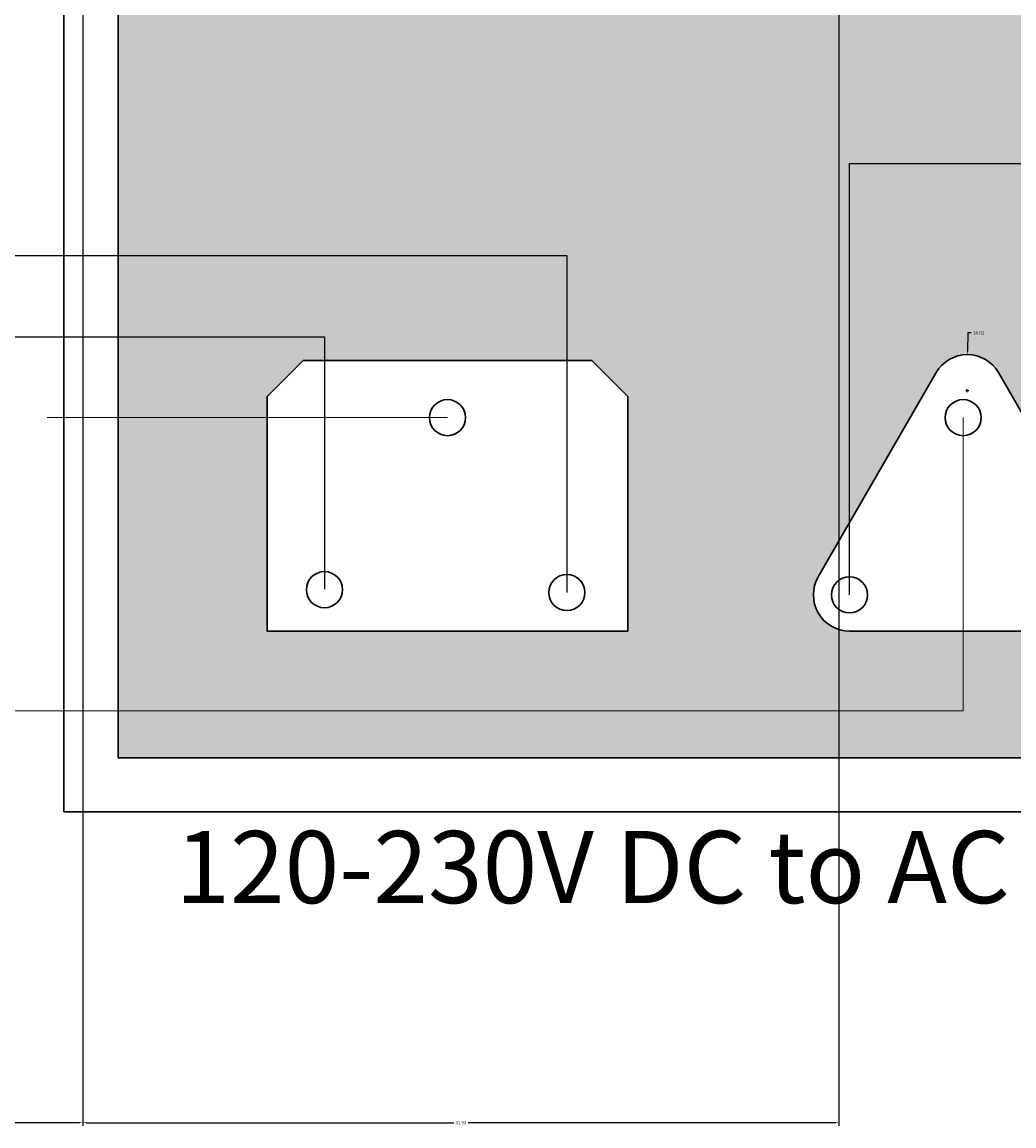
# Model space of a CAD drawing. Units: millimetres. Extents: x -8 to 285, y 5 to 221.
# Tile 17 of 30: x 186 to 241, y 5 to 66. Entities that reach past the tile are written whole.
import ezdxf

# ---------------------------------------------------------------- set-up
doc = ezdxf.new("R2010")
doc.units = ezdxf.units.MM
for name, color, linetype, lineweight in [('A-ANNO-DIMS', 2, 'Continuous', 18), ('E-ANNO-TEXT', 7, 'Continuous', 18), ('E-EQPM-PATT', 252, 'Continuous', 13), ('E-POWR-AC-NEUT', 3, 'Continuous', 25), ('E-POWR-DC-NEG', 3, 'Continuous', 25), ('E-POWR-INVR', 7, 'Continuous', 30)]:
    doc.layers.add(name, color=color, linetype=linetype, lineweight=lineweight)
doc.layers.add('E-POWR-DC-POS', color=30, linetype='Continuous', lineweight=25, true_color=0xf26722)
doc.styles.get("Standard").update_dxf_attribs({"font": 'arial.ttf'})
doc.dimstyles.get("Standard").update_dxf_attribs({"dimtxt": 0.18, "dimasz": 0.18, "dimexe": 0.18, "dimexo": 0.0625, "dimgap": 0.09, "dimtad": 0, "dimtih": 1, "dimtoh": 1, "dimdec": 4, "dimzin": 0, "dimdsep": 46, "dimtxsty": 'Standard', "dimcen": 0.09, "dimadec": 0, "dimazin": 0, "dimtfac": 1, "dimtdec": 4, "dimtofl": 0, "dimtmove": 0, "dimatfit": 3, "dimfxl": 1, "dimtolj": 1, "dimtzin": 0, "dimarcsym": 0})

# ---------------------------------------------------------------- blocks, each defined once
blk = doc.blocks.new('*D13')
at = {"layer": 'A-ANNO-DIMS', "color": 0, "lineweight": -2, "transparency": 16777216}
for p, q in [((145.21, 137.013), (145.21, 5.222)), ((189.039, 137.013), (189.039, 5.222)), ((145.39, 5.402), (166.727, 5.402)), ((188.859, 5.402), (167.522, 5.402))]:
    blk.add_line(p, q, dxfattribs=at)
at = {"layer": 'A-ANNO-DIMS', "color": 0, "transparency": 16777216}
for points in [[(145.39, 5.432), (145.39, 5.372), (145.21, 5.402)], [(188.859, 5.432), (188.859, 5.372), (189.039, 5.402)]]:
    blk.add_solid(points, dxfattribs=at)
at = {"layer": 'Defpoints', "color": 0, "transparency": 16777216}
for p in [(145.21, 137.075), (189.039, 137.075), (189.039, 5.402)]:
    blk.add_point(p, dxfattribs=at)
at = {"layer": 'A-ANNO-DIMS', "color": 0, "transparency": 16777216, "insert": (167.124, 5.402), "char_height": 0.18, "attachment_point": 5}
blk.add_mtext('\\A1;43.83', dxfattribs=at)
blk = doc.blocks.new('*D14')
at = {"layer": 'A-ANNO-DIMS', "color": 0, "lineweight": -2, "transparency": 16777216}
for p, q in [((189.039, 137.013), (189.039, 5.222)), ((230.967, 137.013), (230.967, 5.222)), ((189.219, 5.402), (209.606, 5.402)), ((230.787, 5.402), (210.4, 5.402))]:
    blk.add_line(p, q, dxfattribs=at)
at = {"layer": 'A-ANNO-DIMS', "color": 0, "transparency": 16777216}
for points in [[(189.219, 5.432), (189.219, 5.372), (189.039, 5.402)], [(230.787, 5.432), (230.787, 5.372), (230.967, 5.402)]]:
    blk.add_solid(points, dxfattribs=at)
at = {"layer": 'Defpoints', "color": 0, "transparency": 16777216}
for p in [(189.039, 137.075), (230.967, 137.075), (230.967, 5.402)]:
    blk.add_point(p, dxfattribs=at)
at = {"layer": 'A-ANNO-DIMS', "color": 0, "transparency": 16777216, "insert": (210.003, 5.402), "char_height": 0.18, "attachment_point": 5}
blk.add_mtext('\\A1;41.93', dxfattribs=at)
blk = doc.blocks.new('*D37')
at = {"layer": 'A-ANNO-DIMS', "color": 0, "lineweight": -2, "transparency": 16777216}
for p, q in [((238.11, 49.172), (238.101, 48.152)), ((238.29, 49.172), (238.11, 49.172)), ((237.993, 45.972), (238.173, 45.972)), ((238.083, 45.882), (238.083, 46.062))]:
    blk.add_line(p, q, dxfattribs=at)
at = {"layer": 'A-ANNO-DIMS', "color": 0, "transparency": 16777216}
blk.add_solid([(238.071, 48.152), (238.131, 48.151), (238.1, 47.972)], dxfattribs=at)
at = {"layer": 'Defpoints', "color": 0, "transparency": 16777216}
for p in [(238.1, 47.972), (238.083, 45.972)]:
    blk.add_point(p, dxfattribs=at)
at = {"layer": 'A-ANNO-DIMS', "color": 0, "transparency": 16777216, "insert": (238.718, 49.172), "char_height": 0.18, "attachment_point": 5}
blk.add_mtext('\\A1;3X R2', dxfattribs=at)

msp = doc.modelspace()

# ---------------------------------------------------------------- hatches: boundary and pattern name
at = {"layer": 'E-EQPM-PATT'}
h = msp.add_hatch(color=256, dxfattribs=at)
h.set_gradient(color1=(175, 217, 170), color2=(175, 217, 170), tint=1)
h.paths.add_polyline_path([(255.6152, 99.7021), (190.9955, 99.7021), (190.9955, 53.4644), (215.8749, 53.4644), (215.8749, 47.6512), (217.2608, 47.6512), (219.2608, 45.6512), (219.2608, 32.6512), (199.2608, 32.6512), (199.2608, 44.4759), (190.9955, 44.4759), (190.9955, 28.2311), (237.8513, 28.2311), (237.8513, 32.6512), (231.5468, 32.6512, -0.5773503), (229.8147, 35.6512), (231.5468, 38.6512), (231.5468, 58.5666), (255.6152, 58.5666)])
h.paths.add_polyline_path([(208.2775, 92.6953), (238.0827, 92.6953), (238.0827, 67.6708), (208.2775, 67.6708)], flags=16)
h.paths.add_polyline_path([(213.1801, 80.183, -1), (233.1801, 80.183, -1)], flags=0)
h.paths.add_polyline_path([(215.1801, 80.183, -1), (231.1801, 80.183, -1)], flags=0)
h.paths.add_polyline_path([(217.1801, 80.183, -1), (229.1801, 80.183, -1)], flags=0)
h.paths.add_polyline_path([(219.1801, 80.183, -1), (227.1801, 80.183, -1)], flags=0)
h.paths.add_polyline_path([(255.6152, 58.5666), (231.5468, 58.5666), (231.5468, 38.6512), (236.3506, 46.9717, -0.5773503), (239.8147, 46.9717), (244.6186, 38.6512), (244.6186, 49.925), (255.6152, 49.925)], flags=17)
h.paths.add_polyline_path([(215.8749, 53.4644), (190.9955, 53.4644), (190.9955, 48.962), (202.4345, 48.962), (202.4345, 47.6512), (215.8749, 47.6512)], flags=17)
h.paths.add_polyline_path([(255.6152, 49.925), (244.6186, 49.925), (244.6186, 38.6512), (246.3506, 35.6512, -0.5773503), (244.6186, 32.6512), (237.8513, 32.6512), (237.8513, 28.2311), (190.9955, 28.2311), (190.9955, 25.6297), (255.6152, 25.6297)])
h.paths.add_polyline_path([(199.2608, 45.6512), (201.2608, 47.6512), (202.4345, 47.6512), (202.4345, 48.962), (190.9955, 48.962), (190.9955, 44.4759), (199.2608, 44.4759)], flags=17)

# ---------------------------------------------------------------- linework, layer by layer
at = {"layer": 'E-ANNO-TEXT'}
msp.add_line((209.2608, 44.4759), (187.0614, 44.4759), dxfattribs=at)
msp.add_lwpolyline([(237.8513, 44.4759), (237.8513, 28.2311), (180.7415, 28.2311)], dxfattribs=at)
at = {"layer": 'E-POWR-AC-NEUT'}
msp.add_lwpolyline([(231.5468, 34.6512), (231.5468, 58.5666), (262.873, 58.5666), (262.873, 115.1427), (144.6762, 115.1427), (144.6762, 130.9614)], dxfattribs=at)
at = {"layer": 'E-POWR-DC-NEG'}
for p, q in [((58.1717, 53.4644), (215.8749, 53.4644)), ((215.8749, 53.4644), (215.8749, 34.7803))]:
    msp.add_line(p, q, dxfattribs=at)
at = {"layer": 'E-POWR-DC-POS'}
msp.add_lwpolyline([(52.1717, 48.962), (202.4345, 48.962), (202.4345, 34.9746)], dxfattribs=at)
at = {"layer": 'E-POWR-INVR'}
for points in [[(187.9955, 102.7021), (258.6152, 102.7021), (258.6152, 22.6297), (187.9955, 22.6297)], [(190.9955, 99.7021), (255.6152, 99.7021), (255.6152, 25.6297), (190.9955, 25.6297)], [(201.2608, 47.6512), (217.2608, 47.6512), (219.2608, 45.6512), (219.2608, 32.6512), (199.2608, 32.6512), (199.2608, 45.6512)]]:
    msp.add_lwpolyline(points, close=True, dxfattribs=at)
msp.add_lwpolyline([(239.8147, 46.9717), (246.3506, 35.6512, -0.5773503), (244.6186, 32.6512), (231.5468, 32.6512, -0.5773503), (229.8147, 35.6512), (236.3506, 46.9717)], format="xyb", dxfattribs=at)
for centre in [(209.2608, 44.4759), (237.8513, 44.4759), (202.4345, 34.9422), (215.8749, 34.7803), (231.5468, 34.6512)]:
    msp.add_circle(centre, 1, dxfattribs=at)
msp.add_arc((238.0827, 45.9717), 2, 30, 150, dxfattribs=at)

# ---------------------------------------------------------------- texts
at = {"layer": 'E-ANNO-TEXT', "insert": (194.1702, 21.5692), "char_height": 4, "attachment_point": 1}
msp.add_mtext_dynamic_manual_height_columns('120-230V DC to AC inverter', width=74.08228, gutter_width=12.5, heights=[0], dxfattribs=at)

# ---------------------------------------------------------------- dimensions: what is measured, and where the dimension line sits
at = {"layer": 'A-ANNO-DIMS'}
for base, p1, p2, picture, middle in [((189.039, 5.402), (145.2095, 137.0752), (189.039, 137.0752), '*D13', (167.1243, 5.402)), ((230.9672, 5.402), (189.039, 137.0752), (230.9672, 137.0752), '*D14', (210.0031, 5.402))]:
    dim = msp.add_linear_dim(base=base, p1=p1, p2=p2, dimstyle='Standard', override={"dimdec": 2, "dimlfac": 1, "dimrnd": 0, "dimzin": 0, "dimdsep": 46, "dimlunit": 2}, dxfattribs=at)
    dim.commit()
    dim.dimension.update_dxf_attribs({"geometry": picture, "text_midpoint": middle})
dim = msp.add_radius_dim(center=(238.0827, 45.9717), mpoint=(238.0998, 47.9717), text='3X <>', dimstyle='Standard', override={"dimdec": 0, "dimlfac": 1, "dimrnd": 0, "dimzin": 0, "dimdsep": 46, "dimlunit": 2}, dxfattribs=at)
dim.commit()
dim.dimension.update_dxf_attribs({"geometry": '*D37', "text_midpoint": (238.7175, 49.1716), "dimtype": 164})

doc.saveas('drawing.dxf')
